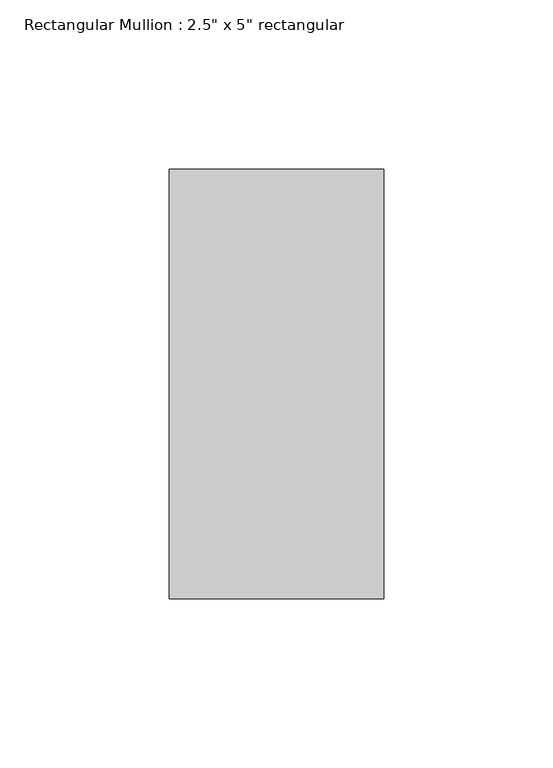
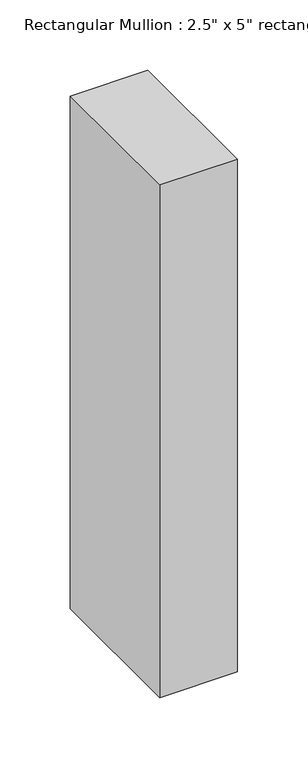
"""IFC4 building model written with IfcOpenShell, lengths in millimetres: member geometry."""

from ifc_helpers import new_model, si_unit, frame, origin, place, context, project, spatial, polyline, outline, extrude, source, transform, mapped, element, save


def member_718fe5d9(model_context):
    return source(origin(), model_context, "Body", "SweptSolid", [
        extrude(outline(polyline([(31.75, 63.5), (31.75, -63.5), (-31.75, -63.5), (-31.75, 63.5), (31.75, 63.5)])), frame((0.0, 0.0, -444.5), z_axis=(0.0, 0.0, 1.0), x_axis=(1.0, 0.0, 0.0)), (0.0, 0.0, 1.0), 444.5),
    ])


if __name__ == "__main__":
    model = new_model("IFC4")
    model_context = context("Model", 3, world=origin())
    ifc_project = project(units=[si_unit("LENGTHUNIT", "METRE", prefix="MILLI")], contexts=[model_context])
    site = spatial("IfcSite", under=ifc_project)
    building = spatial("IfcBuilding", under=site)
    placement = place(None, origin())
    member_shape = member_718fe5d9(model_context)
    element("IfcMember", 1, ObjectType="Rectangular Mullion : 2.5\" x 5\" rectangular", at=placement, inside=building, context=model_context, shape_type="MappedRepresentation", body=[
        mapped(member_shape, transform((0.0, 0.0, 0.0), x_axis=(1.0, 0.0, 0.0), y_axis=(0.0, 1.0, 0.0), z_axis=(0.0, 0.0, 1.0))),
    ])
    save(model, "model.ifc")

# Revit data of these elements
# Type "Rectangular Mullion : 2.5\" x 5\" rectangular"
#   built-in parameter 1007304 = 0.416667 (stored number, unit not read)
#   built-in parameter 1007301 = 0.104167 (stored number, unit not read)
#   built-in parameter 1007300 = 0.104167 (stored number, unit not read)
